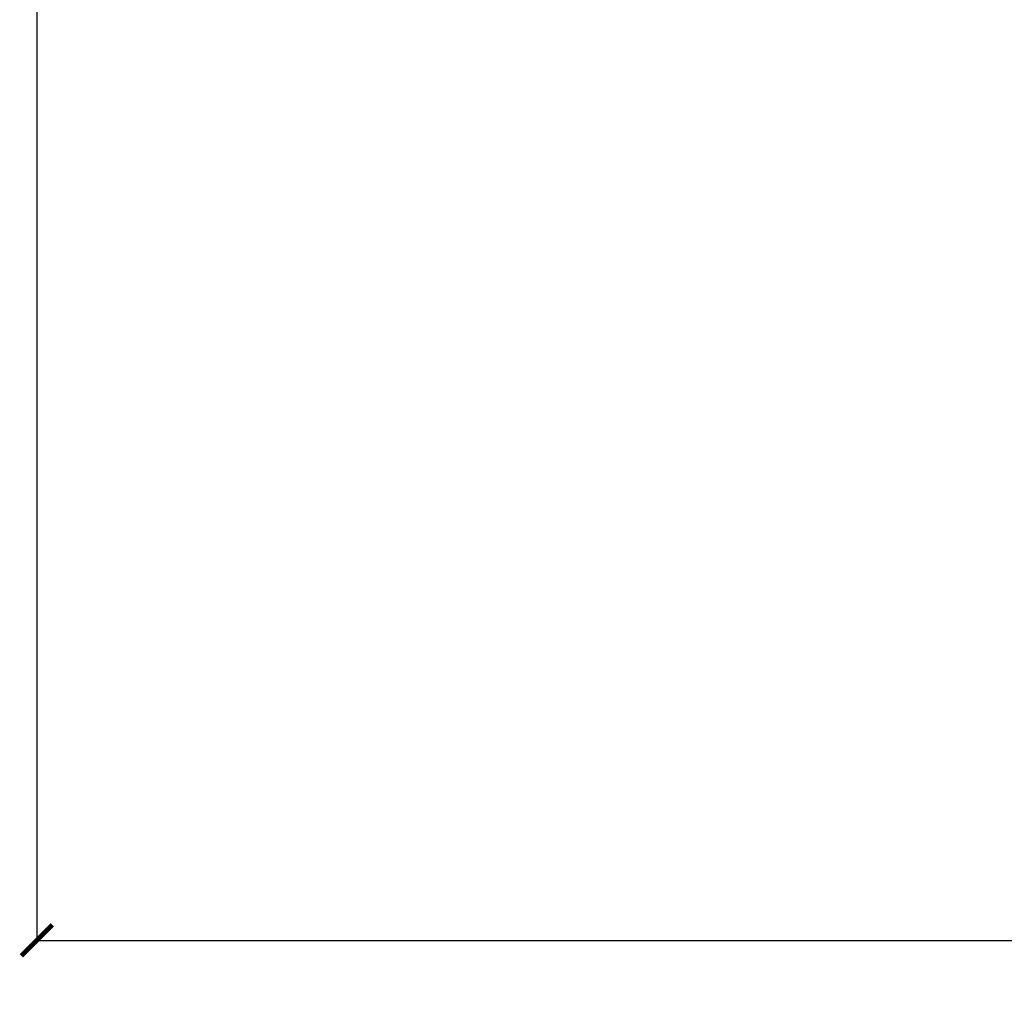
# Model space of a CAD drawing. Units: inches. Extents: x 1704 to 6393, y -157 to 1172.
# Tile 1 of 122: x 1897 to 1961, y -69 to -5. Entities that reach past the tile are written whole.
import ezdxf

# ---------------------------------------------------------------- set-up
doc = ezdxf.new("R2010")
doc.units = ezdxf.units.IN
doc.header["$MEASUREMENT"] = 0
doc.layers.add('A-ANNO-DIMS', color=7, linetype='Continuous', lineweight=13)
doc.styles.get("Standard").update_dxf_attribs({"font": 'arial.ttf'})
doc.dimstyles.get("Standard").update_dxf_attribs({"dimtxt": 6, "dimasz": 2, "dimexe": 0.18, "dimexo": 0.0625, "dimgap": 0.09, "dimtad": 0, "dimtih": 1, "dimtoh": 1, "dimdec": 1, "dimzin": 0, "dimdsep": 46, "dimlunit": 3, "dimtxsty": 'Standard', "dimblk": 'ARCHTICK', "dimcen": 0.09, "dimadec": 0, "dimazin": 0, "dimtfac": 1, "dimtdec": 1, "dimtofl": 0, "dimtmove": 0, "dimatfit": 3, "dimfxl": 1, "dimtolj": 1, "dimtzin": 0, "dimarcsym": 0})

# ---------------------------------------------------------------- blocks, each defined once
blk = doc.blocks.new('_ArchTick')
at = {"color": 0, "linetype": 'ByBlock', "const_width": 0.15}
blk.add_lwpolyline([(-0.5, -0.5), (0.5, 0.5)], dxfattribs=at)
blk = doc.blocks.new('*D90')
at = {"layer": 'A-ANNO-DIMS', "color": 0, "lineweight": -2, "transparency": 16777216}
for p, q in [((1898.349, -3.85), (1898.349, -64.967)), ((2723.349, -3.85), (2723.349, -64.967)), ((1898.349, -64.787), (2304.104, -64.787)), ((2723.349, -64.787), (2317.593, -64.787))]:
    blk.add_line(p, q, dxfattribs=at)
at = {"layer": 'Defpoints', "color": 0, "lineweight": -3, "transparency": 16777216}
for p in [(1898.349, -3.787), (2723.349, -3.787), (2723.349, -64.787)]:
    blk.add_point(p, dxfattribs=at)
at = {"layer": 'A-ANNO-DIMS', "color": 0, "lineweight": -2, "transparency": 16777216, "xscale": 2, "yscale": 2, "zscale": 2, "rotation": 180}
blk.add_blockref('_ArchTick', (1898.349, -64.787), dxfattribs=at)
at = {"layer": 'A-ANNO-DIMS', "color": 0, "lineweight": -2, "transparency": 16777216, "xscale": 2, "yscale": 2, "zscale": 2}
blk.add_blockref('_ArchTick', (2723.349, -64.787), dxfattribs=at)
at = {"layer": 'A-ANNO-DIMS', "color": 0, "transparency": 16777216, "insert": (2310.849, -64.787), "char_height": 6, "attachment_point": 5}
blk.add_mtext('\\A1;825', dxfattribs=at)

msp = doc.modelspace()

# ---------------------------------------------------------------- dimensions: what is measured, and where the dimension line sits
at = {"layer": 'A-ANNO-DIMS'}
dim = msp.add_linear_dim(base=(2723.349, -64.787), p1=(1898.349, -3.787), p2=(2723.349, -3.787), dimstyle='Standard', override={"dimdec": 0, "dimlfac": 1, "dimrnd": 0, "dimzin": 0, "dimdsep": 46, "dimlunit": 2}, dxfattribs=at)
dim.commit()
dim.dimension.update_dxf_attribs({"geometry": '*D90', "text_midpoint": (2310.849, -64.787)})

doc.saveas('drawing.dxf')
